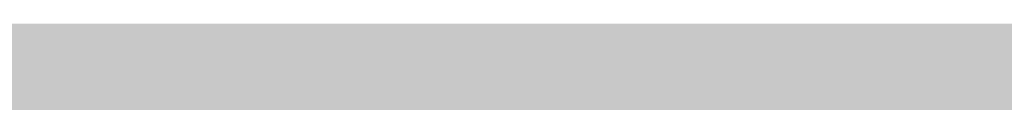
# Model space of a CAD drawing. Units: feet. Extents: x 3168 to 4724, y 827 to 1477.
# Tile 30 of 256: x 3261.901 to 3270.273, y 1098.344 to 1099.001. Entities that reach past the tile are written whole.
import ezdxf

# ---------------------------------------------------------------- set-up
doc = ezdxf.new("R2010")
doc.units = ezdxf.units.FT
doc.layers.add('A-ELEV', color=7, linetype='Continuous', lineweight=35)
doc.layers.add('A-ELEV-PATT', color=8, linetype='Continuous', lineweight=13)

msp = doc.modelspace()

# ---------------------------------------------------------------- hatches: boundary and pattern name
at = {"layer": 'A-ELEV-PATT'}
h = msp.add_hatch(color=256, dxfattribs=at)
h.dxf.hatch_style = 1
edge = h.paths.add_edge_path()
edge.add_ellipse((3552.9058, 979.2201), major_axis=(36.7449, 0), ratio=0.4848485, start_angle=0, end_angle=360)
edge = h.paths.add_edge_path()
edge.add_ellipse((3559.8916, 929.2523), major_axis=(36.7449, 0), ratio=0.4848485, start_angle=0, end_angle=360)
edge = h.paths.add_edge_path()
edge.add_line((3299.3168, 1198.6061), (3479.9167, 1198.6061))
edge.add_line((3479.9167, 1198.6061), (3479.9167, 1209.8686))
edge.add_spline(control_points=[(3479.9167, 1209.8686), (3464.3012, 1209.8686), (3448.6856, 1209.8686), (3410.9491, 1209.8686), (3388.8282, 1209.8686), (3355.6469, 1209.8686), (3344.5864, 1209.8686), (3327.9957, 1209.8686), (3322.4655, 1209.8686), (3314.1702, 1209.8686), (3311.4051, 1209.8686), (3307.2574, 1209.8686), (3305.8748, 1209.8686), (3303.801, 1209.8686), (3303.1097, 1209.8686), (3302.0728, 1209.8686), (3301.7272, 1209.8686), (3301.2087, 1209.8686), (3301.0359, 1209.8686), (3300.7767, 1209.8686), (3300.6903, 1209.8686), (3300.5606, 1209.8686), (3300.5174, 1209.8686), (3300.4526, 1209.8686), (3300.431, 1209.8686), (3300.3986, 1209.8686), (3300.3878, 1209.8686), (3300.3662, 1209.8686), (3300.3457, 1209.8686), (3300.3455, 1209.8686), (3300.3455, 1209.8686), (3300.3433, 1209.8686), (3300.3411, 1209.8686), (3300.3379, 1209.8686), (3300.3368, 1209.8686), (3300.3339, 1209.8686), (3300.3321, 1209.8686), (3300.3255, 1209.8686), (3300.3207, 1209.8686), (3300.3109, 1209.8686), (3300.306, 1209.8686), (3300.2905, 1209.8686), (3300.28, 1209.8686), (3300.2324, 1209.8688), (3300.1953, 1209.869), (3299.9511, 1209.8706), (3299.7448, 1209.8743), (3299.4368, 1209.8833), (3299.3344, 1209.8868), (3299.1811, 1209.8929), (3299.13, 1209.8951), (3298.6522, 1209.9168), (3298.2295, 1209.9457), (3297.6016, 1210.0024), (3297.3934, 1210.0235), (3297.0827, 1210.0583), (3296.9793, 1210.0705), (3296.293, 1210.1549), (3295.7181, 1210.2434), (3294.8687, 1210.3989), (3294.5877, 1210.4545), (3294.1693, 1210.5433), (3294.0304, 1210.5739), (3291.7071, 1211.1012), (3289.6536, 1211.8134), (3285.7763, 1213.564), (3283.9514, 1214.6035), (3280.5122, 1216.9801), (3278.8972, 1218.3176), (3276.3799, 1220.8295), (3275.416, 1221.9177), (3274.0393, 1223.7077), (3273.581, 1224.3495), (3273.1432, 1225.0163)], knot_values=[39.119033, 39.119033, 39.119033, 39.119033, 39.286353, 39.286353, 39.523379, 39.523379, 39.641892, 39.641892, 39.701148, 39.701148, 39.730777, 39.730777, 39.745591, 39.745591, 39.752998, 39.752998, 39.756701, 39.756701, 39.758553, 39.758553, 39.759479, 39.759479, 39.759942, 39.759942, 39.760173, 39.760173, 39.760289, 39.760289, 39.760405, 39.760405, 39.760463, 39.760463, 39.763389, 39.763389, 39.764851, 39.764851, 39.767304, 39.767304, 39.773825, 39.773825, 39.78057, 39.78057, 39.79477, 39.79477, 39.845194, 39.845194, 40.126715, 40.126715, 40.267476, 40.267476, 40.337856, 40.337856, 40.927023, 40.927023, 41.221606, 41.221606, 41.368898, 41.368898, 42.202622, 42.202622, 42.619485, 42.619485, 42.827916, 42.827916, 46.118323, 46.118323, 49.408731, 49.408731, 52.699139, 52.699139, 54.927489, 54.927489, 56.104228, 56.104228, 56.104228, 56.104228], weights=[1, 1, 1, 1, 1, 1, 1, 1, 1, 1, 1, 1, 1, 1, 1, 1, 1, 1, 1, 1, 1, 1, 1, 1, 1, 1, 1, 1, 1, 1, 1, 1, 1, 1, 1, 1, 1, 1, 1, 1, 1, 1, 1, 1, 1, 1, 1, 1, 1, 1, 1, 1, 1, 1, 1, 1, 1, 1, 1, 1, 1, 1, 1, 1, 1, 1, 1, 1, 1, 1, 1, 1, 1, 1], degree=3, periodic=0)
edge.add_line((3273.1432, 1225.0163), (3273.1432, 1099.0163))
edge.add_line((3273.1432, 1099.0163), (3299.3168, 1099.0163))
edge.add_line((3299.3168, 1099.0163), (3299.3168, 1198.6061))
edge = h.paths.add_edge_path()
edge.add_line((3304.7584, 1324.1581), (3479.9167, 1324.1581))
edge.add_line((3479.9167, 1324.1581), (3479.9167, 1335.7146))
edge.add_line((3479.9167, 1335.7146), (3269.1616, 1335.7146))
edge.add_spline(control_points=[(3269.1616, 1335.7146), (3264.0242, 1335.7146), (3258.3641, 1328.9582), (3259.2643, 1323.9003)], knot_values=[0, 0, 0, 0, 15.412191, 15.412191, 15.412191, 15.412191], degree=3, periodic=0)
edge.add_line((3259.2643, 1323.9003), (3265.5168, 1288.7691))
edge.add_line((3265.5168, 1288.7691), (3275.2651, 1261.5456))
edge.add_line((3275.2651, 1261.5456), (3304.7584, 1261.5456))
edge.add_line((3304.7584, 1261.5456), (3304.7584, 1324.1581))
h = msp.add_hatch(color=256, dxfattribs=at)
h.dxf.hatch_style = 1
h.paths.add_polyline_path([(3384.5252, 1099.0163), (3335.0292, 1099.0163), (3299.3168, 1099.0163), (3273.1432, 1099.0163), (3217.5654, 1099.0163), (3168.0693, 827.1163), (3335.0292, 827.1163)])

# ---------------------------------------------------------------- linework, layer by layer
at = {"layer": 'A-ELEV'}
msp.add_open_spline([(3808.5202, 1099.0163), (3808.5202, 1141.4132), (3808.5202, 1183.8102), (3808.5202, 1226.6353), (3808.5202, 1227.0636), (3808.5202, 1227.4918), (3811.4919, 1248.9947), (3814.4635, 1270.4975), (3817.4652, 1292.2176), (3817.4952, 1292.4348), (3817.5253, 1292.652), (3817.5728, 1310.1067), (3817.6203, 1327.5615), (3817.6679, 1345.0163), (3817.6679, 1345.458), (3817.6679, 1345.8996), (3817.6679, 1346.456), (3817.6679, 1346.5708), (3817.6679, 1346.7529), (3817.6679, 1346.8201), (3817.6679, 1346.9349), (3817.6679, 1346.9823), (3817.6679, 1347.0386), (3817.6679, 1347.0474), (3817.6679, 1347.0737), (3817.6679, 1347.0593), (3817.6679, 1347.0615), (3817.6679, 1347.0627), (3817.6679, 1347.066), (3817.6679, 1347.0683), (3817.6679, 1347.075), (3817.6679, 1347.0795), (3817.6678, 1347.0929), (3817.6678, 1347.1019), (3817.6678, 1347.1288), (3817.6677, 1347.1467), (3817.6674, 1347.2004), (3817.6672, 1347.2362), (3817.6661, 1347.3434), (3817.665, 1347.4147), (3817.6608, 1347.6281), (3817.6566, 1347.7697), (3817.64, 1348.1925), (3817.6235, 1348.4716), (3817.5591, 1349.3001), (3817.4961, 1349.8406), (3817.2554, 1351.4242), (3817.0263, 1352.4288), (3816.3069, 1354.8889), (3815.7437, 1356.2687), (3814.464, 1358.8192), (3813.7464, 1359.991), (3812.1958, 1362.1723), (3811.3622, 1363.1821), (3809.5888, 1365.069), (3808.6488, 1365.9461), (3806.6543, 1367.5796), (3805.5997, 1368.3362), (3803.3529, 1369.7223), (3802.1605, 1370.3524), (3799.6008, 1371.4536), (3798.2327, 1371.9255), (3795.2801, 1372.6346), (3793.6931, 1372.8721), (3791.8694, 1372.9265), (3791.7409, 1372.9292), (3791.3534, 1372.9341), (3791.0927, 1372.9329), (3790.3041, 1372.9151), (3789.7695, 1372.8842), (3789.2092, 1372.8302), (3789.1906, 1372.8284), (3789.1349, 1372.8229), (3789.0977, 1372.8191), (3789.0484, 1372.814), (3789.0364, 1372.8127), (3789.0003, 1372.8089), (3788.9761, 1372.8063), (3788.9494, 1372.8034), (3788.9468, 1372.8031), (3788.9426, 1372.8027), (3788.941, 1372.8025), (3788.9386, 1372.8022), (3788.9378, 1372.8021), (3788.9354, 1372.8019), (3788.8675, 1372.7944), (3788.7569, 1372.7822), (3788.7015, 1372.7761), (3788.5355, 1372.7579), (3788.4249, 1372.7457), (3788.0929, 1372.7092), (3787.8715, 1372.6848), (3787.2075, 1372.6118), (3786.7648, 1372.5631), (3785.4368, 1372.417), (3784.5515, 1372.3196), (3781.8954, 1372.0274), (3780.1247, 1371.8327), (3774.8126, 1371.2483), (3771.2713, 1370.8587), (3760.6471, 1369.69), (3753.5643, 1368.9109), (3732.316, 1366.5735), (3718.1504, 1365.0152), (3694.0068, 1362.3593), (3684.0287, 1361.2617), (3674.0506, 1360.1641), (3664.6007, 1360.1641), (3655.1508, 1360.1641), (3626.8011, 1360.1641), (3607.9013, 1360.1641), (3551.2019, 1360.1641), (3513.4023, 1360.1641), (3467.7252, 1360.1641), (3459.8476, 1360.1641), (3436.2149, 1360.1641), (3420.4597, 1360.1641), (3373.1943, 1360.1641), (3341.6839, 1360.1641), (3302.8482, 1360.1641), (3295.5227, 1360.1641), (3286.0383, 1360.1641), (3283.8794, 1360.1641), (3277.4026, 1360.1641), (3273.0848, 1360.1641), (3267.7329, 1360.1641), (3266.6988, 1360.1641), (3263.5965, 1360.1641), (3261.5284, 1360.1641), (3259.2369, 1360.1641), (3259.0137, 1360.1641), (3258.344, 1360.1641), (3257.8975, 1360.1641), (3257.431, 1360.1641), (3257.411, 1360.1641), (3257.3706, 1360.1641), (3257.3755, 1360.1641), (3257.3746, 1360.1641), (3257.3739, 1360.1641), (3257.372, 1360.1641), (3257.3706, 1360.1641), (3257.3667, 1360.1641), (3257.364, 1360.1641), (3257.3561, 1360.1641), (3257.3508, 1360.164), (3257.335, 1360.164), (3257.3244, 1360.164), (3257.2928, 1360.1639), (3257.2717, 1360.1638), (3257.2084, 1360.1634), (3257.1663, 1360.163), (3257.0402, 1360.1614), (3256.9563, 1360.1598), (3256.7055, 1360.1534), (3256.5392, 1360.147), (3256.0436, 1360.1219), (3255.7173, 1360.0971), (3254.7524, 1360.0005), (3254.128, 1359.9065), (3252.1801, 1359.5253), (3250.9416, 1359.144), (3248.6702, 1358.2433), (3247.6357, 1357.7238), (3245.7326, 1356.6035), (3244.8634, 1356.0021), (3243.2531, 1354.7429), (3242.512, 1354.0847), (3240.7511, 1352.3448), (3239.801, 1351.2296), (3238.0878, 1348.8724), (3237.3247, 1347.6304), (3235.9825, 1344.9716), (3235.4022, 1343.5549), (3234.5911, 1340.8155), (3234.3109, 1339.5435), (3233.9765, 1336.8026), (3233.9221, 1335.3309), (3234.1489, 1332.5913), (3234.3495, 1331.3672), (3234.7199, 1329.9994), (3234.7524, 1329.8834), (3234.8536, 1329.5348), (3234.9259, 1329.3017), (3235.0248, 1329.0026), (3235.0469, 1328.9369), (3235.0776, 1328.8472), (3235.0859, 1328.8232), (3235.1109, 1328.7511), (3235.1278, 1328.703), (3235.148, 1328.6462), (3235.1511, 1328.6376), (3235.1561, 1328.6235), (3235.1581, 1328.618), (3235.1602, 1328.612), (3235.1656, 1328.5969), (3235.1801, 1328.5565), (3235.1903, 1328.5281), (3235.2208, 1328.4429), (3235.2411, 1328.3862), (3235.3021, 1328.2159), (3235.3427, 1328.1023), (3235.4647, 1327.7617), (3235.546, 1327.5346), (3235.79, 1326.8534), (3235.9526, 1326.3992), (3236.4405, 1325.0367), (3236.7657, 1324.1284), (3237.7415, 1321.4034), (3238.392, 1319.5868), (3240.3435, 1314.1369), (3241.6445, 1310.5036), (3245.5476, 1299.6037), (3248.1496, 1292.3371), (3255.9557, 1270.5374), (3261.1598, 1256.0042), (3267.3876, 1238.612), (3268.4114, 1235.7529), (3269.5104, 1232.6839), (3269.5856, 1232.4739), (3269.7066, 1232.1359), (3269.7524, 1232.0079), (3269.8273, 1231.7987), (3269.8564, 1231.7176), (3269.9063, 1231.5781), (3269.9272, 1231.5198), (3269.9725, 1231.3934), (3269.9968, 1231.3254), (3270.0265, 1231.2425), (3270.0318, 1231.2277), (3270.0403, 1231.204), (3270.0392, 1231.207), (3270.0394, 1231.2066), (3270.0394, 1231.2064), (3270.0396, 1231.2058), (3270.0398, 1231.2055), (3270.0402, 1231.2043), (3270.0404, 1231.2036), (3270.0413, 1231.2013), (3270.0418, 1231.1998), (3270.0434, 1231.1953), (3270.0445, 1231.1922), (3270.0478, 1231.1832), (3270.0499, 1231.1771), (3270.0564, 1231.159), (3270.0608, 1231.147), (3270.0739, 1231.1108), (3270.0826, 1231.0867), (3270.1089, 1231.0144), (3270.1266, 1230.9663), (3270.1799, 1230.8225), (3270.2159, 1230.7269), (3270.3253, 1230.4415), (3270.4, 1230.2528), (3270.6292, 1229.6914), (3270.7889, 1229.3235), (3271.2865, 1228.2383), (3271.6431, 1227.5398), (3272.7759, 1225.5153), (3273.6142, 1224.2605), (3275.416, 1221.9177), (3276.3799, 1220.8295), (3278.8972, 1218.3176), (3280.5122, 1216.9801), (3283.9514, 1214.6035), (3285.7763, 1213.564), (3289.6536, 1211.8134), (3291.7071, 1211.1012), (3294.0304, 1210.5739), (3294.1693, 1210.5433), (3294.5877, 1210.4545), (3294.8687, 1210.3989), (3295.7181, 1210.2434), (3296.293, 1210.1549), (3296.9793, 1210.0705), (3297.0827, 1210.0583), (3297.3934, 1210.0235), (3297.6016, 1210.0024), (3298.2295, 1209.9457), (3298.6522, 1209.9168), (3299.13, 1209.8951), (3299.1811, 1209.8929), (3299.3344, 1209.8868), (3299.4368, 1209.8833), (3299.7448, 1209.8743), (3299.9511, 1209.8706), (3300.1953, 1209.869), (3300.2324, 1209.8688), (3300.28, 1209.8686), (3300.2905, 1209.8686), (3300.306, 1209.8686), (3300.3109, 1209.8686), (3300.3207, 1209.8686), (3300.3255, 1209.8686), (3300.3321, 1209.8686), (3300.3339, 1209.8686), (3300.3368, 1209.8686), (3300.3379, 1209.8686), (3300.3411, 1209.8686), (3300.3433, 1209.8686), (3300.3455, 1209.8686), (3300.3455, 1209.8686), (3300.3457, 1209.8686), (3300.3662, 1209.8686), (3300.3878, 1209.8686), (3300.3986, 1209.8686), (3300.431, 1209.8686), (3300.4526, 1209.8686), (3300.5174, 1209.8686), (3300.5606, 1209.8686), (3300.6903, 1209.8686), (3300.7767, 1209.8686), (3301.0359, 1209.8686), (3301.2087, 1209.8686), (3301.7272, 1209.8686), (3302.0728, 1209.8686), (3303.1097, 1209.8686), (3303.801, 1209.8686), (3305.8748, 1209.8686), (3307.2574, 1209.8686), (3311.4051, 1209.8686), (3314.1702, 1209.8686), (3322.4655, 1209.8686), (3327.9957, 1209.8686), (3344.5864, 1209.8686), (3355.6469, 1209.8686), (3388.8282, 1209.8686), (3410.9491, 1209.8686), (3477.3119, 1209.8686), (3521.5537, 1209.8686), (3566.8362, 1209.8686), (3567.8769, 1209.8686), (3570.999, 1209.8686), (3573.0804, 1209.8686), (3575.7814, 1209.8686), (3576.4009, 1209.8686), (3577.2958, 1209.8686), (3577.5712, 1209.8686), (3578.3971, 1209.8686), (3578.9478, 1209.8686), (3579.7565, 1209.8686), (3580.0145, 1209.8686), (3580.3427, 1209.8686), (3580.3269, 1209.8686), (3580.3272, 1209.8686), (3580.3273, 1209.8686), (3580.3278, 1209.8686), (3580.3281, 1209.8686), (3580.329, 1209.8686), (3580.3296, 1209.8686), (3580.3314, 1209.8686), (3580.3327, 1209.8686), (3580.3363, 1209.8686), (3580.3388, 1209.8686), (3580.3461, 1209.8686), (3580.351, 1209.8686), (3580.3657, 1209.8685), (3580.3754, 1209.8685), (3580.4048, 1209.8684), (3580.4244, 1209.8684), (3580.4832, 1209.8681), (3580.5224, 1209.8678), (3580.6404, 1209.8666), (3580.7192, 1209.8655), (3580.9563, 1209.8608), (3581.1152, 1209.8561), (3581.5942, 1209.8372), (3581.9164, 1209.8183), (3582.8899, 1209.7424), (3583.548, 1209.6662), (3585.5318, 1209.3606), (3586.8672, 1209.0539), (3589.4715, 1208.2525), (3590.7402, 1207.7579), (3591.9955, 1207.1588), (3592.0578, 1207.1287), (3592.2442, 1207.038), (3592.3677, 1206.9766), (3592.7353, 1206.7904), (3592.9768, 1206.6631), (3593.2445, 1206.5164), (3593.2747, 1206.4998), (3593.3651, 1206.4498), (3593.4251, 1206.4163), (3593.6043, 1206.3153), (3593.7227, 1206.2472), (3593.8572, 1206.1684), (3593.8744, 1206.1583), (3593.9257, 1206.128), (3593.9599, 1206.1078), (3594.0621, 1206.0469), (3594.1298, 1206.0061), (3594.2084, 1205.9582), (3594.2197, 1205.9513), (3594.2534, 1205.9307), (3594.2758, 1205.9169), (3594.343, 1205.8755), (3594.3876, 1205.8479), (3594.4336, 1205.819), (3594.4353, 1205.818), (3594.4402, 1205.8149), (3594.4435, 1205.8129), (3594.4471, 1205.8106), (3594.4475, 1205.8103), (3594.4487, 1205.8096), (3594.4495, 1205.8091), (3594.4504, 1205.8086), (3594.4505, 1205.8085), (3594.4506, 1205.8084), (3594.4674, 1205.7979), (3594.4933, 1205.7817), (3594.5062, 1205.7736), (3594.545, 1205.7492), (3594.5709, 1205.733), (3594.6485, 1205.6844), (3594.7002, 1205.652), (3594.8554, 1205.5547), (3594.9589, 1205.4898), (3595.2694, 1205.2953), (3595.4763, 1205.1656), (3596.0972, 1204.7765), (3596.5111, 1204.5171), (3597.7528, 1203.7388), (3598.5807, 1203.22), (3601.0642, 1201.6636), (3602.7198, 1200.6259), (3607.6868, 1197.513), (3610.9981, 1195.4377), (3620.932, 1189.2119), (3627.5546, 1185.0614), (3647.4225, 1172.6097), (3660.6678, 1164.3086), (3700.4035, 1139.4053), (3726.894, 1122.8031), (3757.2057, 1103.8061), (3761.027, 1101.4112), (3764.8482, 1099.0163), (3745.3283, 1099.0163), (3725.8083, 1099.0163), (3706.2884, 1099.0163), (3706.2884, 1108.4532), (3706.2884, 1117.8902), (3706.2884, 1127.3271), (3710.7508, 1127.3271), (3715.2131, 1127.3271), (3719.6755, 1127.3271)], degree=3, knots=[0, 0, 0, 0, 0.982037, 0.982037, 0.991957, 0.991957, 0.991957, 1.966522, 1.966522, 1.976367, 1.976367, 1.976367, 2.976367, 2.976367, 2.976367, 3.00169, 3.00169, 3.008272, 3.008272, 3.012129, 3.012129, 3.014851, 3.014851, 3.015353, 3.015353, 3.016359, 3.016359, 3.017365, 3.017365, 3.019376, 3.019376, 3.023398, 3.023398, 3.031442, 3.031442, 3.047531, 3.047531, 3.079708, 3.079708, 3.144063, 3.144063, 3.272772, 3.272772, 3.53019, 3.53019, 4.045026, 4.045026, 5.074698, 5.074698, 6.700878, 6.700878, 8.327058, 8.327058, 9.953238, 9.953238, 11.579418, 11.579418, 13.205598, 13.205598, 14.831778, 14.831778, 16.457958, 16.457958, 18.084138, 18.084138, 18.206872, 18.206872, 18.45234, 18.45234, 18.943275, 18.943275, 18.960093, 18.960093, 18.993729, 18.993729, 19.00461, 19.00461, 19.026374, 19.026374, 19.028737, 19.028737, 19.03018, 19.03018, 19.030897, 19.030897, 19.032332, 19.032332, 19.033766, 19.033766, 19.036636, 19.036636, 19.042374, 19.042374, 19.053851, 19.053851, 19.076805, 19.076805, 19.122714, 19.122714, 19.21453, 19.21453, 19.398163, 19.398163, 19.765429, 19.765429, 20.024128, 20.024128, 20.024128, 20.092031, 20.092031, 20.227836, 20.227836, 20.499446, 20.499446, 20.556051, 20.556051, 20.66926, 20.66926, 20.895678, 20.895678, 20.948316, 20.948316, 20.963829, 20.963829, 20.994855, 20.994855, 21.002285, 21.002285, 21.017146, 21.017146, 21.01875, 21.01875, 21.021959, 21.021959, 21.022102, 21.022102, 21.022249, 21.022249, 21.022708, 21.022708, 21.023627, 21.023627, 21.025464, 21.025464, 21.029138, 21.029138, 21.036486, 21.036486, 21.051183, 21.051183, 21.080575, 21.080575, 21.139361, 21.139361, 21.256932, 21.256932, 21.492073, 21.492073, 21.962356, 21.962356, 23.01002, 23.01002, 24.057684, 24.057684, 25.105348, 25.105348, 26.153011, 26.153011, 27.776787, 27.776787, 29.400562, 29.400562, 31.024337, 31.024337, 32.278801, 32.278801, 33.533265, 33.533265, 34.467568, 34.467568, 34.553971, 34.553971, 34.726776, 34.726776, 34.775309, 34.775309, 34.793079, 34.793079, 34.82862, 34.82862, 34.834979, 34.834979, 34.839039, 34.839039, 34.839411, 34.839411, 34.840285, 34.840285, 34.842034, 34.842034, 34.845531, 34.845531, 34.852525, 34.852525, 34.866512, 34.866512, 34.894488, 34.894488, 34.950439, 34.950439, 35.062342, 35.062342, 35.286147, 35.286147, 35.733758, 35.733758, 35.821815, 35.821815, 35.828283, 35.828283, 35.832225, 35.832225, 35.834724, 35.834724, 35.836521, 35.836521, 35.838617, 35.838617, 35.839073, 35.839073, 35.839345, 35.839345, 35.839617, 35.839617, 35.840161, 35.840161, 35.841249, 35.841249, 35.843425, 35.843425, 35.847778, 35.847778, 35.856482, 35.856482, 35.873891, 35.873891, 35.908709, 35.908709, 35.978345, 35.978345, 36.117617, 36.117617, 36.396161, 36.396161, 36.953248, 36.953248, 38.067423, 38.067423, 40.295772, 40.295772, 42.524122, 42.524122, 45.81453, 45.81453, 49.104937, 49.104937, 52.395345, 52.395345, 52.603776, 52.603776, 53.020639, 53.020639, 53.854363, 53.854363, 54.001655, 54.001655, 54.296238, 54.296238, 54.885405, 54.885405, 54.955785, 54.955785, 55.096546, 55.096546, 55.378067, 55.378067, 55.42849, 55.42849, 55.442691, 55.442691, 55.449436, 55.449436, 55.455957, 55.455957, 55.458409, 55.458409, 55.459872, 55.459872, 55.462798, 55.462798, 55.462856, 55.462856, 55.462972, 55.462972, 55.463088, 55.463088, 55.463319, 55.463319, 55.463782, 55.463782, 55.464708, 55.464708, 55.46656, 55.46656, 55.470263, 55.470263, 55.47767, 55.47767, 55.492484, 55.492484, 55.522112, 55.522112, 55.581369, 55.581369, 55.699882, 55.699882, 55.936907, 55.936907, 56.410959, 56.410959, 56.42211, 56.42211, 56.444413, 56.444413, 56.451051, 56.451051, 56.454001, 56.454001, 56.459901, 56.459901, 56.462666, 56.462666, 56.463418, 56.463418, 56.464171, 56.464171, 56.465675, 56.465675, 56.468684, 56.468684, 56.474702, 56.474702, 56.486738, 56.486738, 56.51081, 56.51081, 56.558955, 56.558955, 56.655243, 56.655243, 56.847821, 56.847821, 57.232975, 57.232975, 58.003284, 58.003284, 59.543901, 59.543901, 62.625137, 62.625137, 68.787607, 68.787607, 74.950078, 74.950078, 75.27336, 75.27336, 75.919923, 75.919923, 77.213051, 77.213051, 77.377769, 77.377769, 77.707206, 77.707206, 78.366079, 78.366079, 78.462532, 78.462532, 78.655436, 78.655436, 79.041245, 79.041245, 79.105735, 79.105735, 79.234714, 79.234714, 79.492672, 79.492672, 79.502197, 79.502197, 79.521249, 79.521249, 79.523534, 79.523534, 79.528103, 79.528103, 79.528682, 79.528682, 79.528885, 79.528885, 79.529089, 79.529089, 79.529495, 79.529495, 79.530308, 79.530308, 79.531935, 79.531935, 79.535187, 79.535187, 79.541693, 79.541693, 79.554704, 79.554704, 79.580725, 79.580725, 79.632769, 79.632769, 79.736856, 79.736856, 79.94503, 79.94503, 80.361377, 80.361377, 80.421435, 80.421435, 80.421435, 81.421435, 81.421435, 81.421435, 82.421435, 82.421435, 82.421435, 83.421435, 83.421435, 83.421435, 83.421435], dxfattribs=at)

doc.saveas('drawing.dxf')
